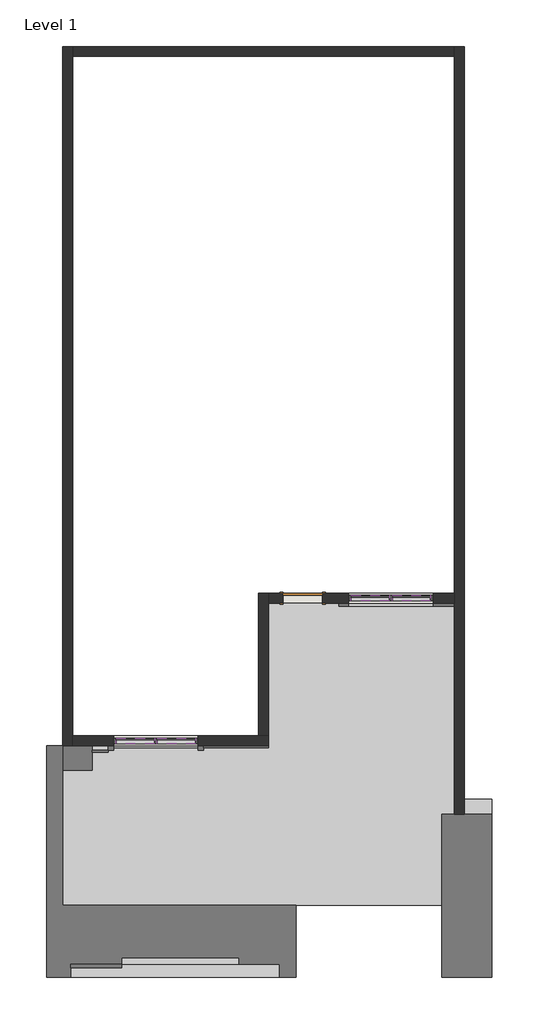
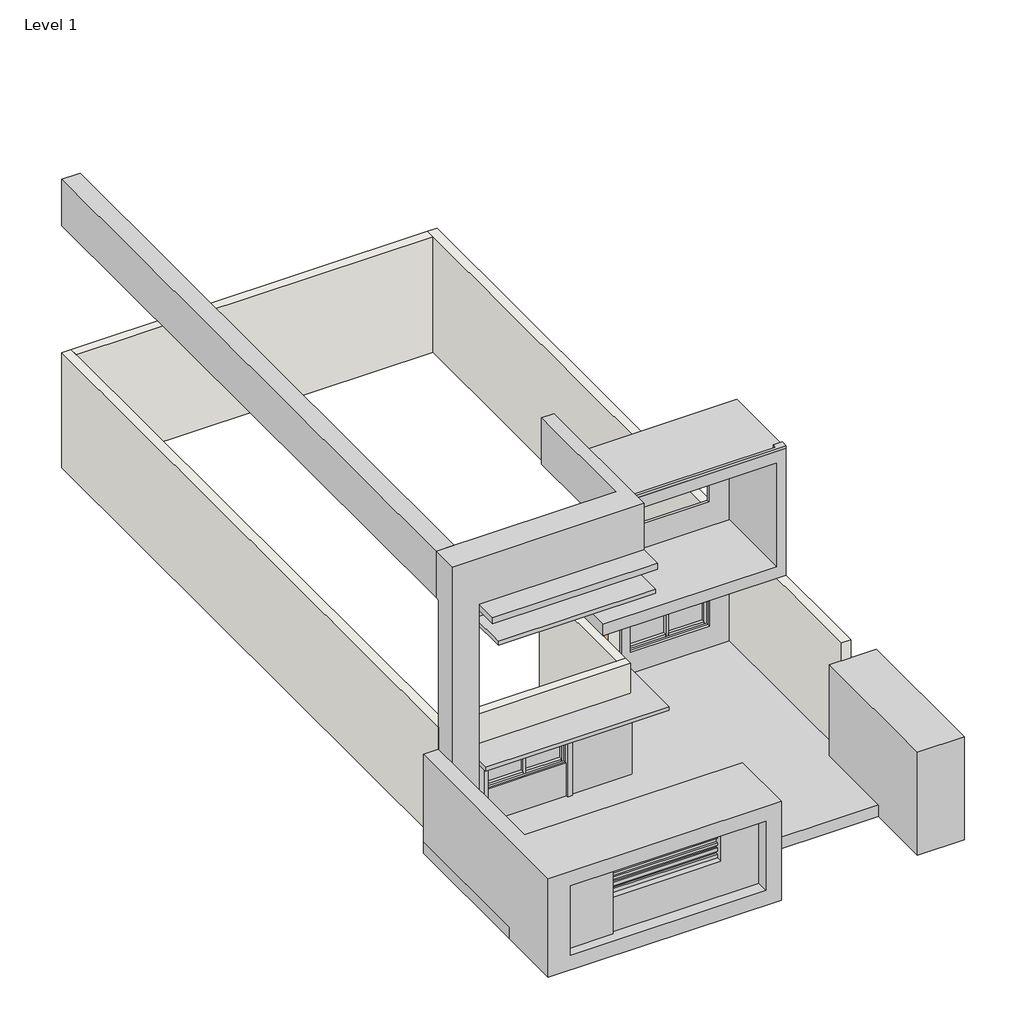
# One storey: 14 members, 6 walls, 4 plates, 1 door, 1 proxy.
"""IFC4 building model written with IfcOpenShell, lengths in millimetres."""

from ifc_helpers import new_model, si_unit, frame, origin, origin_with_axes, place, context, project, spatial, polyline, outline, extrude, faceted_brep, transform, mapped, element, save
from components import generic_models_1_generic_models_1_aa7367fc, door_0ca8825f, member_f1f71bde, member_7034f759, member_55de22a4, member_9b0ed4fb, member_83f53977, system_panel_glazed_014df054, system_panel_glazed_1adc8ad2

model = new_model("IFC4")

# Units and contexts
model_context = context("Model", 3, world=origin())
ifc_project = project(units=[si_unit("LENGTHUNIT", "METRE", prefix="MILLI")], contexts=[model_context])

# Site, building, storey
site = spatial("IfcSite", under=ifc_project)
building = spatial("IfcBuilding", under=site)
storey = spatial("IfcBuildingStorey", under=building, Name="Level 1", Elevation=0.0)

# Proxy
placement = place(None, origin())
generic_models_1_generic_models_1_shape = generic_models_1_generic_models_1_aa7367fc(model_context)
element("IfcBuildingElementProxy", 1, Name="Generic Models 1 : Generic Models 1", ObjectType="Generic Models 1 : Generic Models 1", at=placement, inside=storey, context=model_context, shape_type="MappedRepresentation", body=[
    mapped(generic_models_1_generic_models_1_shape, transform((0.0, 0.0, 0.0), x_axis=(1.0, 0.0, 0.0), y_axis=(0.0, 1.0, 0.0), z_axis=(0.0, 0.0, 1.0))),
])

# Door
door_shape = door_0ca8825f(model_context)
element("IfcDoor", 2, ObjectType="Single-Flush : 36\" x 84\"", at=placement, inside=storey, context=model_context, shape_type="MappedRepresentation", body=[
    mapped(door_shape, transform((-14492.3161422, -7377.2867758, 101.6), x_axis=(1.0, 0.0, 0.0), y_axis=(0.0, 1.0, 0.0), z_axis=(0.0, 0.0, 1.0))),
])

# Members
member_shape = member_f1f71bde(model_context)
element("IfcMember", 3, ObjectType="Rectangular Mullion : 2.5\" x 5\" rectangular", at=placement, inside=storey, context=model_context, shape_type="MappedRepresentation", body=[
    mapped(member_shape, transform((-17889.5661422, -10704.6867758, 1025.0994511), x_axis=(0.0, 0.0, -1.0), y_axis=(0.0, -1.0, 0.0), z_axis=(-1.0, 0.0, 0.0))),
])
element("IfcMember", 4, ObjectType="Rectangular Mullion : 2.5\" x 5\" rectangular", at=placement, inside=storey, context=model_context, shape_type="MappedRepresentation", body=[
    mapped(member_shape, transform((-18848.4161422, -10704.6867758, 1025.0994511), x_axis=(0.0, 0.0, -1.0), y_axis=(0.0, -1.0, 0.0), z_axis=(-1.0, 0.0, 0.0))),
])
element("IfcMember", 5, ObjectType="Rectangular Mullion : 2.5\" x 5\" rectangular", at=placement, inside=storey, context=model_context, shape_type="MappedRepresentation", body=[
    mapped(member_shape, transform((-12403.1661422, -7377.2867758, 714.2961729), x_axis=(0.0, 0.0, -1.0), y_axis=(0.0, -1.0, 0.0), z_axis=(-1.0, 0.0, 0.0))),
])
element("IfcMember", 6, ObjectType="Rectangular Mullion : 2.5\" x 5\" rectangular", at=placement, inside=storey, context=model_context, shape_type="MappedRepresentation", body=[
    mapped(member_shape, transform((-13362.0161422, -7377.2867758, 714.2961729), x_axis=(0.0, 0.0, -1.0), y_axis=(0.0, -1.0, 0.0), z_axis=(-1.0, 0.0, 0.0))),
])
member_2_shape = member_7034f759(model_context)
element("IfcMember", 7, ObjectType="Rectangular Mullion : 2.5\" x 5\" rectangular", at=placement, inside=storey, context=model_context, shape_type="MappedRepresentation", body=[
    mapped(member_2_shape, transform((-17921.3161422, -10704.6867758, 1025.0994511), x_axis=(1.0, 0.0, 0.0), y_axis=(0.0, -1.0, 0.0), z_axis=(0.0, 0.0, -1.0))),
])
element("IfcMember", 8, ObjectType="Rectangular Mullion : 2.5\" x 5\" rectangular", at=placement, inside=storey, context=model_context, shape_type="MappedRepresentation", body=[
    mapped(member_shape, transform((-17953.0661422, -10704.6867758, 2163.0020846), x_axis=(0.0, 0.0, 1.0), y_axis=(0.0, -1.0, 0.0), z_axis=(1.0, 0.0, 0.0))),
])
element("IfcMember", 9, ObjectType="Rectangular Mullion : 2.5\" x 5\" rectangular", at=placement, inside=storey, context=model_context, shape_type="MappedRepresentation", body=[
    mapped(member_shape, transform((-16994.2161422, -10704.6867758, 2163.0020846), x_axis=(0.0, 0.0, 1.0), y_axis=(0.0, -1.0, 0.0), z_axis=(1.0, 0.0, 0.0))),
])
element("IfcMember", 10, ObjectType="Rectangular Mullion : 2.5\" x 5\" rectangular", at=placement, inside=storey, context=model_context, shape_type="MappedRepresentation", body=[
    mapped(member_shape, transform((-12466.6661422, -7377.2867758, 2217.8846358), x_axis=(0.0, 0.0, 1.0), y_axis=(0.0, -1.0, 0.0), z_axis=(1.0, 0.0, 0.0))),
])
element("IfcMember", 11, ObjectType="Rectangular Mullion : 2.5\" x 5\" rectangular", at=placement, inside=storey, context=model_context, shape_type="MappedRepresentation", body=[
    mapped(member_shape, transform((-11507.8161422, -7377.2867758, 2217.8846358), x_axis=(0.0, 0.0, 1.0), y_axis=(0.0, -1.0, 0.0), z_axis=(1.0, 0.0, 0.0))),
])
member_3_shape = member_55de22a4(model_context)
element("IfcMember", 12, ObjectType="Rectangular Mullion : 2.5\" x 5\" rectangular", at=placement, inside=storey, context=model_context, shape_type="MappedRepresentation", body=[
    mapped(member_3_shape, transform((-18911.9161422, -10704.6867758, 2163.0020846), x_axis=(-1.0, 0.0, 0.0), y_axis=(0.0, -1.0, 0.0), z_axis=(0.0, 0.0, 1.0))),
])
element("IfcMember", 13, ObjectType="Rectangular Mullion : 2.5\" x 5\" rectangular", at=placement, inside=storey, context=model_context, shape_type="MappedRepresentation", body=[
    mapped(member_3_shape, transform((-16930.7161422, -10704.6867758, 1025.0994511), x_axis=(1.0, 0.0, 0.0), y_axis=(0.0, -1.0, 0.0), z_axis=(0.0, 0.0, -1.0))),
])
member_4_shape = member_9b0ed4fb(model_context)
element("IfcMember", 14, ObjectType="Rectangular Mullion : 2.5\" x 5\" rectangular", at=placement, inside=storey, context=model_context, shape_type="MappedRepresentation", body=[
    mapped(member_4_shape, transform((-12434.9161422, -7377.2867758, 714.2961729), x_axis=(1.0, 0.0, 0.0), y_axis=(0.0, -1.0, 0.0), z_axis=(0.0, 0.0, -1.0))),
])
member_5_shape = member_83f53977(model_context)
element("IfcMember", 15, ObjectType="Rectangular Mullion : 2.5\" x 5\" rectangular", at=placement, inside=storey, context=model_context, shape_type="MappedRepresentation", body=[
    mapped(member_5_shape, transform((-13425.5161422, -7377.2867758, 2217.8846358), x_axis=(-1.0, 0.0, 0.0), y_axis=(0.0, -1.0, 0.0), z_axis=(0.0, 0.0, 1.0))),
])
element("IfcMember", 16, ObjectType="Rectangular Mullion : 2.5\" x 5\" rectangular", at=placement, inside=storey, context=model_context, shape_type="MappedRepresentation", body=[
    mapped(member_5_shape, transform((-11444.3161422, -7377.2867758, 714.2961729), x_axis=(1.0, 0.0, 0.0), y_axis=(0.0, -1.0, 0.0), z_axis=(0.0, 0.0, -1.0))),
])

# Plates
system_panel_glazed_shape = system_panel_glazed_014df054(model_context)
element("IfcPlate", 17, ObjectType="System Panel : Glazed", at=placement, inside=storey, context=model_context, shape_type="MappedRepresentation", body=[
    mapped(system_panel_glazed_shape, transform((-18400.7411422, -10704.6867758, 1088.5994511), x_axis=(1.0, 0.0, 0.0), y_axis=(0.0, 1.0, 0.0), z_axis=(0.0, 0.0, 1.0))),
])
element("IfcPlate", 18, ObjectType="System Panel : Glazed", at=placement, inside=storey, context=model_context, shape_type="MappedRepresentation", body=[
    mapped(system_panel_glazed_shape, transform((-17441.8911422, -10704.6867758, 1088.5994511), x_axis=(1.0, 0.0, 0.0), y_axis=(0.0, 1.0, 0.0), z_axis=(0.0, 0.0, 1.0))),
])
system_panel_glazed_2_shape = system_panel_glazed_1adc8ad2(model_context)
element("IfcPlate", 19, ObjectType="System Panel : Glazed", at=placement, inside=storey, context=model_context, shape_type="MappedRepresentation", body=[
    mapped(system_panel_glazed_2_shape, transform((-12914.3411422, -7377.2867758, 777.7961729), x_axis=(1.0, 0.0, 0.0), y_axis=(0.0, 1.0, 0.0), z_axis=(0.0, 0.0, 1.0))),
])
element("IfcPlate", 20, ObjectType="System Panel : Glazed", at=placement, inside=storey, context=model_context, shape_type="MappedRepresentation", body=[
    mapped(system_panel_glazed_2_shape, transform((-11955.4911422, -7377.2867758, 777.7961729), x_axis=(1.0, 0.0, 0.0), y_axis=(0.0, 1.0, 0.0), z_axis=(0.0, 0.0, 1.0))),
])

# Walls
element("IfcWall", 21, ObjectType="9\"", at=placement, inside=storey, context=model_context, shape_type="Brep", body=[
    faceted_brep([(-10720.4161422, -12419.1867758, 0.0), (-10720.4161422, 5487.8132242, 0.0), (-10720.4161422, 5487.8132242, 3048.0), (-10720.4161422, -12419.1867758, 3048.0), (-10949.0161422, -12419.1867758, 0.0), (-10949.0161422, -12419.1867758, 3048.0), (-10949.0161422, -7491.5867758, 3048.0), (-10949.0161422, -7262.9867758, 3048.0), (-10949.0161422, 5259.2132242, 3048.0), (-10949.0161422, 5487.8132242, 3048.0), (-10949.0161422, 5487.8132242, 0.0), (-10949.0161422, 5259.2132242, 0.0), (-10949.0161422, -7262.9867758, 0.0), (-10949.0161422, -7491.5867758, 0.0)], [[[0, 1, 2, 3]], [[4, 5, 6, 7, 8, 9, 10, 11, 12, 13]], [[1, 0, 4, 13, 12, 11, 10]], [[3, 2, 9, 8, 7, 6, 5]], [[0, 3, 5, 4]], [[2, 1, 10, 9]]]),
])
element("IfcWall", 22, ObjectType="9\"", at=placement, inside=storey, context=model_context, shape_type="SweptSolid", body=[
    extrude(outline(polyline([(-19864.4161422, 5487.8132242), (-10949.0161422, 5487.8132242), (-10949.0161422, 5259.2132242), (-19864.4161422, 5259.2132242), (-19864.4161422, 5487.8132242)])), origin_with_axes(), (0.0, 0.0, 1.0), 3048.0),
])
element("IfcWall", 23, ObjectType="9\"", at=placement, inside=storey, context=model_context, shape_type="Brep", body=[
    faceted_brep([(-19864.4161422, -10818.9867758, 0.0), (-15292.4161422, -10818.9867758, 0.0), (-15292.4161422, -10818.9867758, 3048.0), (-19864.4161422, -10818.9867758, 3048.0), (-18911.9161422, -10818.9867758, 1025.0994511), (-18911.9161422, -10818.9867758, 2163.0020846), (-16930.7161422, -10818.9867758, 2163.0020846), (-16930.7161422, -10818.9867758, 1025.0994511), (-15292.4161422, -10590.3867758, 0.0), (-15521.0161422, -10590.3867758, 0.0), (-19864.4161422, -10590.3867758, 0.0), (-19864.4161422, -10590.3867758, 3048.0), (-15521.0161422, -10590.3867758, 3048.0), (-15292.4161422, -10590.3867758, 3048.0), (-18911.9161422, -10590.3867758, 2163.0020846), (-18911.9161422, -10590.3867758, 1025.0994511), (-16930.7161422, -10590.3867758, 1025.0994511), (-16930.7161422, -10590.3867758, 2163.0020846)], [[[0, 1, 2, 3], [4, 5, 6, 7]], [[8, 9, 10, 11, 12, 13], [14, 15, 16, 17]], [[1, 0, 10, 9, 8]], [[3, 2, 13, 12, 11]], [[2, 1, 8, 13]], [[4, 15, 14, 5]], [[5, 14, 17, 6]], [[6, 17, 16, 7]], [[15, 4, 7, 16]], [[0, 3, 11, 10]]]),
])
element("IfcWall", 24, ObjectType="9\"", at=placement, inside=storey, context=model_context, shape_type="Brep", body=[
    faceted_brep([(-15292.4161422, -10590.3867758, 0.0), (-15292.4161422, -7491.5867758, 0.0), (-15292.4161422, -7262.9867758, 0.0), (-15292.4161422, -7262.9867758, 3048.0), (-15292.4161422, -7491.5867758, 3048.0), (-15292.4161422, -10590.3867758, 3048.0), (-15521.0161422, -10590.3867758, 0.0), (-15521.0161422, -10590.3867758, 3048.0), (-15521.0161422, -7262.9867758, 3048.0), (-15521.0161422, -7262.9867758, 0.0)], [[[0, 1, 2, 3, 4, 5]], [[6, 7, 8, 9]], [[2, 1, 0, 6, 9]], [[5, 4, 3, 8, 7]], [[0, 5, 7, 6]], [[3, 2, 9, 8]]]),
])
element("IfcWall", 25, ObjectType="9\"", at=placement, inside=storey, context=model_context, shape_type="SweptSolid", body=[
    extrude(outline(polyline([(0.0, -15292.4161422), (0.0, -10949.0161422), (3048.0, -10949.0161422), (3048.0, -15292.4161422), (0.0, -15292.4161422)]), holes=[polyline([(101.6, -14949.5161422), (2235.2, -14949.5161422), (2235.2, -14035.1161422), (101.6, -14035.1161422), (101.6, -14949.5161422)]), polyline([(714.2961729, -13425.5161422), (2217.8846358, -13425.5161422), (2217.8846358, -11444.3161422), (714.2961729, -11444.3161422), (714.2961729, -13425.5161422)])]), frame((0.0, -7491.5867758, 0.0), z_axis=(0.0, 1.0, 0.0), x_axis=(0.0, 0.0, 1.0)), (0.0, 0.0, 1.0), 228.6),
])
element("IfcWall", 26, ObjectType="9\"", at=placement, inside=storey, context=model_context, shape_type="Brep", body=[
    faceted_brep([(-19864.4161422, -10818.9867758, 0.0), (-19864.4161422, -10590.3867758, 0.0), (-19864.4161422, 5259.2132242, 0.0), (-19864.4161422, 5487.8132242, 0.0), (-19864.4161422, 5487.8132242, 3048.0), (-19864.4161422, 5259.2132242, 3048.0), (-19864.4161422, -10590.3867758, 3048.0), (-19864.4161422, -10818.9867758, 3048.0), (-20093.0161422, -10818.9867758, 0.0), (-20093.0161422, -10818.9867758, 3048.0), (-20093.0161422, 5487.8132242, 3048.0), (-20093.0161422, 5487.8132242, 0.0)], [[[0, 1, 2, 3, 4, 5, 6, 7]], [[8, 9, 10, 11]], [[3, 2, 1, 0, 8, 11]], [[7, 6, 5, 4, 10, 9]], [[4, 3, 11, 10]], [[0, 7, 9, 8]]]),
])

save(model, "model.ifc")

# Revit data of these elements
# Type "Single-Flush : 36\" x 84\""
#   Type Mark = "1"
#   Construction Type Id = "MDOOR"
#   Assembly Code = "C1020"
#   Analytic Construction = "Metal"
#   Thickness = 0' - 2"
#   Heat Transfer Coefficient (U) = 0.651978 BTU/(h·ft²·°F)
#   Height = 7' - 0"
#   Trim Projection Ext = 0' - 1"
#   Trim Projection Int = 0' - 1"
#   Trim Width = 0' - 3"
#   Width = 3' - 0"
#   Define Thermal Properties by = 1
#   Define Thermal Properties by = 1
#   Door Material = Door - Panel
#   Frame Material = Door - Frame
#   Visual Light Transmittance = 0
#   Solar Heat Gain Coefficient = 0
#   Function = (empty or 0)
#   Wall Closure = (empty or 0)
# Type "Rectangular Mullion : 2.5\" x 5\" rectangular"
#   built-in parameter 1007304 = 0.416667 (stored number, unit not read)
#   built-in parameter 1007301 = 0.104167 (stored number, unit not read)
#   built-in parameter 1007300 = 0.104167 (stored number, unit not read)
# Type "System Panel : Glazed"
#   Construction Type Id = "GSP4R"
#   Analytic Construction = "1/8 in Pilkington single glazing"
#   Visual Light Transmittance = 0.9
#   Solar Heat Gain Coefficient = 0.86
#   Heat Transfer Coefficient (U) = 1.18115 BTU/(h·ft²·°F)
#   Define Thermal Properties by = 1
# Type "9\""
#   Assembly Code = "B2010"
#   Layers, outside or top first: 0' - 9" no material (function 1)
# Element 1 (IfcBuildingElementProxy, "Generic Models 1 : Generic Models 1")
#   Phase Created = New Construction
# Element 2 (IfcDoor, "Single-Flush : 36\" x 84\"")
#   Phase Created = New Construction
#   Materials on its faces: "Door - Frame", "Door - Panel"
# Elements 3, 4, 5, 6, 7, 8, 9, 10, 11, 12, 13, 14, 15, 16 (IfcMember, "Rectangular Mullion : 2.5\" x 5\" rectangular")
#   Phase Created = New Construction
#   Materials on its faces: "Aluminum"
# Elements 17, 18, 19, 20 (IfcPlate, "System Panel : Glazed")
#   Phase Created = New Construction
#   Materials on its faces: "Glass"
# Elements 21, 22, 23, 24, 25, 26 (IfcWall, "9\"")
#   Top Offset = 0' - 0"
#   Base Offset = 0' - 0"
#   Unconnected Height = 10' - 0"
#   wall height = 10' - 0"
#   Phase Created = New Construction
#   Base Constraint = Level 1
#   Materials on its faces: "Default Wall"
# Materials
#   "Door - Panel": class "Wood", colour RGB 210 159 95, transparency 0, Cost = 0
#   "Door - Frame": colour RGB 118 70 51, transparency 0, Cost = 0
#   "Aluminum": class "Metal", colour RGB 247 247 247, transparency 0, Description = "Aluminum 6061", Cost = 0
#   "Glass": class "Glass", colour RGB 0 128 192, transparency 0.75, Description = "Soda Lime Glass", Cost = 0
#   "Default Wall": colour RGB 128 128 128, transparency 0, Cost = 0
